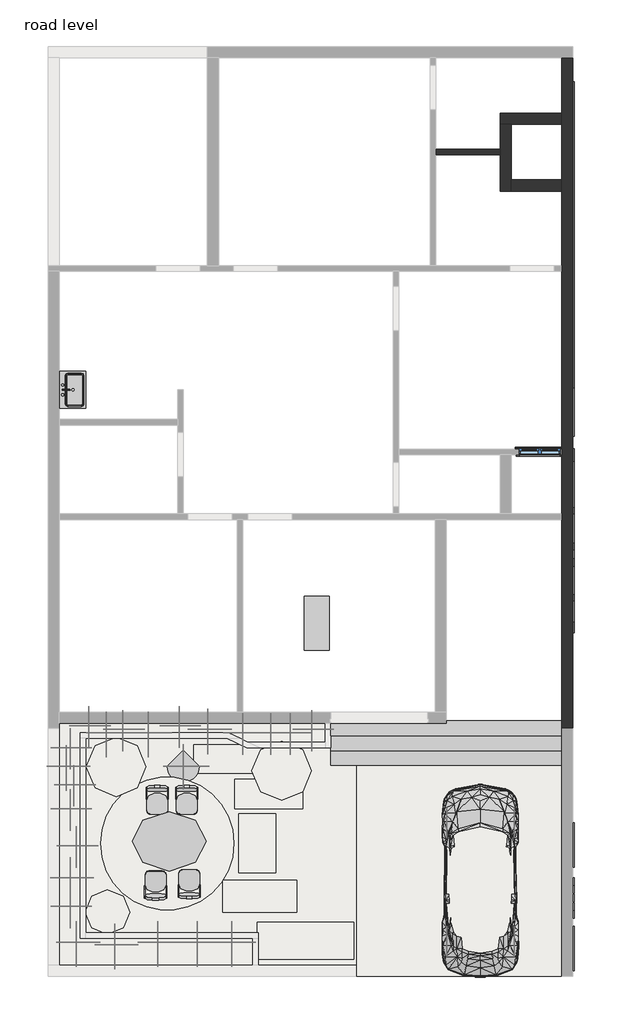
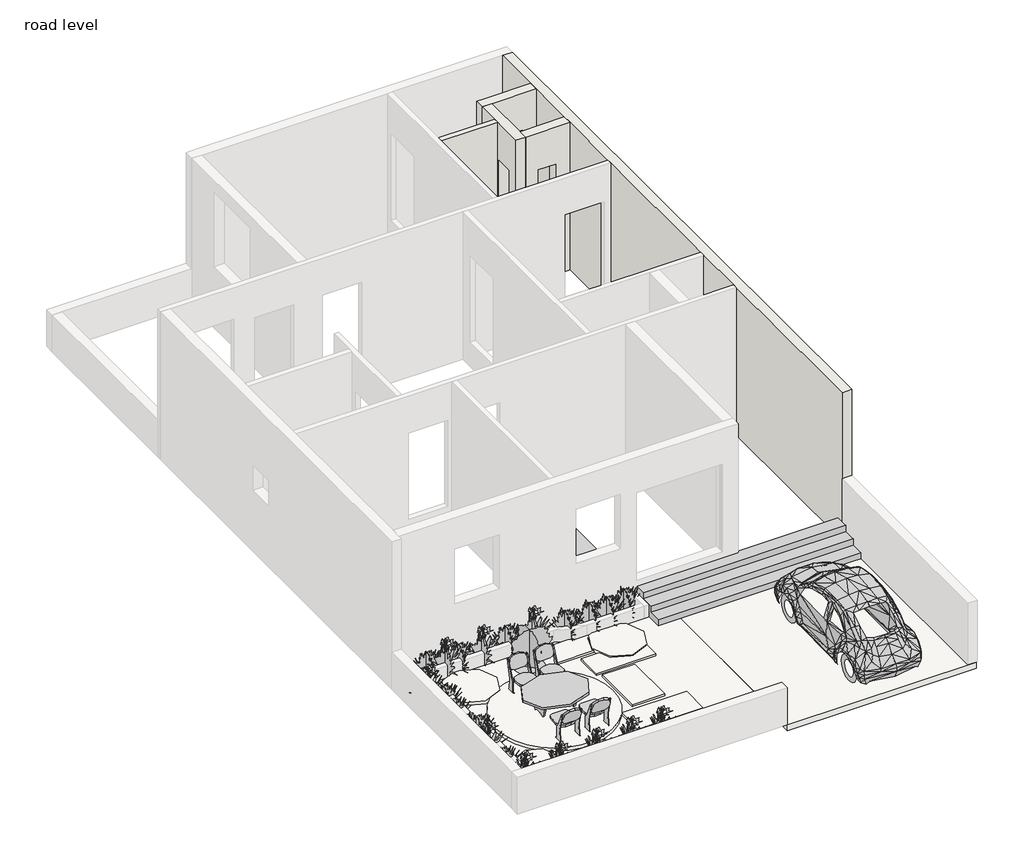
# One storey, part 2 of 2: 23 geographic elements, 9 furniture elements, 7 slabs, 5 proxies, 5 walls, 1 flow terminal, 1 window.
"""IFC4 building model written with IfcOpenShell, lengths in millimetres."""

from ifc_helpers import new_model, si_unit, point, frame, frame_2d, origin, origin_with_axes, place, context, project, spatial, polyline, circle_curve, trimmed, segment, composite_curve, outline, extrude, faceted_brep, transform, mapped, element, save
from components import muntin_pattern_2x2_muntin_pattern_2x2_b3fe6957, muntin_pattern_2x2_muntin_pattern_2x2_3e0ecaf2, rpc_beetle_rpc_beetle_31f8b51e, trim_window_exterior_flat_with_sill_41619996, trim_window_interior_flat_picture_frame_51c85655, flow_terminal_4d548711, casework_1_casework_1_eb7a94e5, casework_2_casework_2_b74305db, casework_3_casework_3_5667240a, furniture_eb3a3c23, furniture_74675f9f, furniture_c105135d, rpc_plant_tropical_55f6ff97, rpc_plant_tropical_dagger_2_80c14bd7, geographic_element_e27c54a3, window_a598f463

model = new_model("IFC4")

# Units and contexts
model_context = context("Model", 3, world=origin())
ifc_project = project(units=[si_unit("LENGTHUNIT", "METRE", prefix="MILLI")], contexts=[model_context])

# Site, building, storey
site = spatial("IfcSite", under=ifc_project)
building = spatial("IfcBuilding", under=site)
storey = spatial("IfcBuildingStorey", under=building, Name="road level", Elevation=0.0)

# Proxies
placement = place(None, origin())
muntin_pattern_2x2_muntin_pattern_2x2_shape = muntin_pattern_2x2_muntin_pattern_2x2_b3fe6957(model_context)
element("IfcBuildingElementProxy", 1, Name="Muntin Pattern_2x2 : Muntin Pattern_2x2", ObjectType="Muntin Pattern_2x2 : Muntin Pattern_2x2", at=placement, inside=storey, context=model_context, shape_type="MappedRepresentation", body=[
    mapped(muntin_pattern_2x2_muntin_pattern_2x2_shape, transform((1784.5376403, 4516.9007925, 984.25), x_axis=(1.0, 0.0, 0.0), y_axis=(0.0, 1.0, 0.0), z_axis=(0.0, 0.0, 1.0))),
])
muntin_pattern_2x2_muntin_pattern_2x2_2_shape = muntin_pattern_2x2_muntin_pattern_2x2_3e0ecaf2(model_context)
element("IfcBuildingElementProxy", 2, Name="Muntin Pattern_2x2 : Muntin Pattern_2x2", ObjectType="Muntin Pattern_2x2 : Muntin Pattern_2x2", at=placement, inside=storey, context=model_context, shape_type="MappedRepresentation", body=[
    mapped(muntin_pattern_2x2_muntin_pattern_2x2_2_shape, transform((2213.1626403, 4516.9007925, 984.25), x_axis=(-1.0, 0.0, 0.0), y_axis=(0.0, -1.0, 0.0), z_axis=(0.0, 0.0, 1.0))),
])
rpc_beetle_rpc_beetle_shape = rpc_beetle_rpc_beetle_31f8b51e(model_context)
element("IfcBuildingElementProxy", 3, Name="RPC Beetle : RPC Beetle", ObjectType="RPC Beetle : RPC Beetle", at=placement, inside=storey, context=model_context, shape_type="MappedRepresentation", body=[
    mapped(rpc_beetle_rpc_beetle_shape, transform((779.6501403, -5586.8025668, 0.0), x_axis=(1.0, 0.0, 0.0), y_axis=(0.0, 1.0, 0.0), z_axis=(0.0, 0.0, 1.0))),
])
trim_window_exterior_flat_with_sill_shape = trim_window_exterior_flat_with_sill_41619996(model_context)
element("IfcBuildingElementProxy", 4, Name="Trim-Window-Exterior-Flat : with Sill", ObjectType="Trim-Window-Exterior-Flat : with Sill", at=placement, inside=storey, context=model_context, shape_type="MappedRepresentation", body=[
    mapped(trim_window_exterior_flat_with_sill_shape, transform((1998.8501403, 4526.4257925, 1828.8), x_axis=(-1.0, 0.0, 0.0), y_axis=(0.0, 0.0, 1.0), z_axis=(0.0, 1.0, 0.0))),
])
trim_window_interior_flat_picture_frame_shape = trim_window_interior_flat_picture_frame_51c85655(model_context)
element("IfcBuildingElementProxy", 5, Name="Trim-Window-Interior-Flat : Picture Frame", ObjectType="Trim-Window-Interior-Flat : Picture Frame", at=placement, inside=storey, context=model_context, shape_type="MappedRepresentation", body=[
    mapped(trim_window_interior_flat_picture_frame_shape, transform((1998.8501403, 4412.1257925, 1828.8), x_axis=(1.0, 0.0, 0.0), y_axis=(0.0, 0.0, 1.0), z_axis=(0.0, -1.0, 0.0))),
])

# Flow terminal
flow_terminal_shape = flow_terminal_4d548711(model_context)
element("IfcFlowTerminal", 6, ObjectType="Sink Kitchen-Single : 30\" x 21\"", at=placement, inside=storey, context=model_context, shape_type="MappedRepresentation", body=[
    mapped(flow_terminal_shape, transform((-7600.0044586, 5729.936552, 0.0), x_axis=(0.0, 1.0, 0.0), y_axis=(-1.0, 0.0, 0.0), z_axis=(0.0, 0.0, 1.0))),
])

# Furniture
casework_1_casework_1_shape = casework_1_casework_1_eb7a94e5(model_context)
element("IfcFurniture", 7, ObjectType="Casework 1 : Casework 1", at=placement, inside=storey, context=model_context, shape_type="MappedRepresentation", body=[
    mapped(casework_1_casework_1_shape, transform((0.0, 0.0, 0.0), x_axis=(1.0, 0.0, 0.0), y_axis=(0.0, 1.0, 0.0), z_axis=(0.0, 0.0, 1.0))),
])
casework_2_casework_2_shape = casework_2_casework_2_b74305db(model_context)
element("IfcFurniture", 8, ObjectType="Casework 2 : Casework 2", at=placement, inside=storey, context=model_context, shape_type="MappedRepresentation", body=[
    mapped(casework_2_casework_2_shape, transform((0.0, 0.0, 0.0), x_axis=(1.0, 0.0, 0.0), y_axis=(0.0, 1.0, 0.0), z_axis=(0.0, 0.0, 1.0))),
])
casework_3_casework_3_shape = casework_3_casework_3_5667240a(model_context)
element("IfcFurniture", 9, ObjectType="Casework 3 : Casework 3", at=placement, inside=storey, context=model_context, shape_type="MappedRepresentation", body=[
    mapped(casework_3_casework_3_shape, transform((0.0, 0.0, 0.0), x_axis=(1.0, 0.0, 0.0), y_axis=(0.0, 1.0, 0.0), z_axis=(0.0, 0.0, 1.0))),
])
furniture_shape = furniture_eb3a3c23(model_context)
element("IfcFurniture", 10, ObjectType="Seating-Auditorium : 18\" x 24\" x 30\"", at=placement, inside=storey, context=model_context, shape_type="MappedRepresentation", body=[
    mapped(furniture_shape, transform((-6061.2777286, -4646.8421746, 76.2), x_axis=(1.0, 0.0, 0.0), y_axis=(0.0, 1.0, 0.0), z_axis=(0.0, 0.0, 1.0))),
])
element("IfcFurniture", 11, ObjectType="Seating-Auditorium : 18\" x 24\" x 30\"", at=placement, inside=storey, context=model_context, shape_type="MappedRepresentation", body=[
    mapped(furniture_shape, transform((-5706.7715198, -2488.6271569, 76.2), x_axis=(-1.0, 0.0, 0.0), y_axis=(0.0, -1.0, 0.0), z_axis=(0.0, 0.0, 1.0))),
])
element("IfcFurniture", 12, ObjectType="Seating-Auditorium : 18\" x 24\" x 30\"", at=placement, inside=storey, context=model_context, shape_type="MappedRepresentation", body=[
    mapped(furniture_shape, transform((-5097.1715198, -2488.6271569, 76.2), x_axis=(-1.0, 0.0, 0.0), y_axis=(0.0, -1.0, 0.0), z_axis=(0.0, 0.0, 1.0))),
])
element("IfcFurniture", 13, ObjectType="Seating-Auditorium : 18\" x 24\" x 30\"", at=placement, inside=storey, context=model_context, shape_type="MappedRepresentation", body=[
    mapped(furniture_shape, transform((-5367.8272575, -4621.4421746, 76.2), x_axis=(1.0, 0.0, 0.0), y_axis=(0.0, 1.0, 0.0), z_axis=(0.0, 0.0, 1.0))),
])
furniture_2_shape = furniture_74675f9f(model_context)
element("IfcFurniture", 14, ObjectType="Table-Coffee Mission : 44\" x 20\"", at=placement, inside=storey, context=model_context, shape_type="MappedRepresentation", body=[
    mapped(furniture_2_shape, transform((-2585.8498597, 945.0257925, 0.0), x_axis=(0.0, 1.0, 0.0), y_axis=(-1.0, 0.0, 0.0), z_axis=(0.0, 0.0, 1.0))),
])
furniture_3_shape = furniture_c105135d(model_context)
element("IfcFurniture", 15, ObjectType="Table-Ellipse : 60\" x 48\"", at=placement, inside=storey, context=model_context, shape_type="MappedRepresentation", body=[
    mapped(furniture_3_shape, transform((-5621.1498597, -3542.5667647, 76.2), x_axis=(1.0, 0.0, 0.0), y_axis=(0.0, 1.0, 0.0), z_axis=(0.0, 0.0, 1.0))),
])

# Geographic elements
rpc_plant_tropical_shape = rpc_plant_tropical_55f6ff97(model_context)
element("IfcGeographicElement", 16, ObjectType="RPC Plant - Tropical", at=placement, inside=storey, context=model_context, shape_type="MappedRepresentation", body=[
    mapped(rpc_plant_tropical_shape, transform((-4330.7993887, -5612.2025668, 0.0), x_axis=(1.0, 0.0, 0.0), y_axis=(0.0, 1.0, 0.0), z_axis=(0.0, 0.0, 1.0))),
])
element("IfcGeographicElement", 17, ObjectType="RPC Plant - Tropical", at=placement, inside=storey, context=model_context, shape_type="MappedRepresentation", body=[
    mapped(rpc_plant_tropical_shape, transform((-5041.9993887, -5612.2025668, 0.0), x_axis=(1.0, 0.0, 0.0), y_axis=(0.0, 1.0, 0.0), z_axis=(0.0, 0.0, 1.0))),
])
element("IfcGeographicElement", 18, ObjectType="RPC Plant - Tropical", at=placement, inside=storey, context=model_context, shape_type="MappedRepresentation", body=[
    mapped(rpc_plant_tropical_shape, transform((-5854.7993887, -5612.2025668, 0.0), x_axis=(1.0, 0.0, 0.0), y_axis=(0.0, 1.0, 0.0), z_axis=(0.0, 0.0, 1.0))),
])
element("IfcGeographicElement", 19, ObjectType="RPC Plant - Tropical", at=placement, inside=storey, context=model_context, shape_type="MappedRepresentation", body=[
    mapped(rpc_plant_tropical_shape, transform((-6743.7993887, -5663.0025668, 0.0), x_axis=(1.0, 0.0, 0.0), y_axis=(0.0, 1.0, 0.0), z_axis=(0.0, 0.0, 1.0))),
])
element("IfcGeographicElement", 20, ObjectType="RPC Plant - Tropical", at=placement, inside=storey, context=model_context, shape_type="MappedRepresentation", body=[
    mapped(rpc_plant_tropical_shape, transform((-7531.1993887, -5612.2025668, 0.0), x_axis=(1.0, 0.0, 0.0), y_axis=(0.0, 1.0, 0.0), z_axis=(0.0, 0.0, 1.0))),
])
element("IfcGeographicElement", 21, ObjectType="RPC Plant - Tropical", at=placement, inside=storey, context=model_context, shape_type="MappedRepresentation", body=[
    mapped(rpc_plant_tropical_shape, transform((-7658.1993887, -4294.0266914, 0.0), x_axis=(1.0, 0.0, 0.0), y_axis=(0.0, 1.0, 0.0), z_axis=(0.0, 0.0, 1.0))),
])
element("IfcGeographicElement", 22, ObjectType="RPC Plant - Tropical", at=placement, inside=storey, context=model_context, shape_type="MappedRepresentation", body=[
    mapped(rpc_plant_tropical_shape, transform((-4827.8987169, -1239.3742075, 0.0), x_axis=(1.0, 0.0, 0.0), y_axis=(0.0, 1.0, 0.0), z_axis=(0.0, 0.0, 1.0))),
])
element("IfcGeographicElement", 23, ObjectType="RPC Plant - Tropical", at=placement, inside=storey, context=model_context, shape_type="MappedRepresentation", body=[
    mapped(rpc_plant_tropical_shape, transform((-6052.9498597, -1309.5266914, 0.0), x_axis=(1.0, 0.0, 0.0), y_axis=(0.0, 1.0, 0.0), z_axis=(0.0, 0.0, 1.0))),
])
element("IfcGeographicElement", 24, ObjectType="RPC Plant - Tropical", at=placement, inside=storey, context=model_context, shape_type="MappedRepresentation", body=[
    mapped(rpc_plant_tropical_shape, transform((-6916.5498597, -1309.5266914, 0.0), x_axis=(1.0, 0.0, 0.0), y_axis=(0.0, 1.0, 0.0), z_axis=(0.0, 0.0, 1.0))),
])
element("IfcGeographicElement", 25, ObjectType="RPC Plant - Tropical", at=placement, inside=storey, context=model_context, shape_type="MappedRepresentation", body=[
    mapped(rpc_plant_tropical_shape, transform((-7734.3993887, -1993.1667647, 0.0), x_axis=(1.0, 0.0, 0.0), y_axis=(0.0, 1.0, 0.0), z_axis=(0.0, 0.0, 1.0))),
])
rpc_plant_tropical_dagger_2_shape = rpc_plant_tropical_dagger_2_80c14bd7(model_context)
element("IfcGeographicElement", 26, ObjectType="RPC Plant - Tropical : Dagger - 2'", at=placement, inside=storey, context=model_context, shape_type="MappedRepresentation", body=[
    mapped(rpc_plant_tropical_dagger_2_shape, transform((-7658.1993887, -4878.2266914, 0.0), x_axis=(1.0, 0.0, 0.0), y_axis=(0.0, 1.0, 0.0), z_axis=(0.0, 0.0, 1.0))),
])
element("IfcGeographicElement", 27, ObjectType="RPC Plant - Tropical : Dagger - 2'", at=placement, inside=storey, context=model_context, shape_type="MappedRepresentation", body=[
    mapped(rpc_plant_tropical_dagger_2_shape, transform((-7531.1993887, -3633.6266914, 0.0), x_axis=(1.0, 0.0, 0.0), y_axis=(0.0, 1.0, 0.0), z_axis=(0.0, 0.0, 1.0))),
])
element("IfcGeographicElement", 28, ObjectType="RPC Plant - Tropical : Dagger - 2'", at=placement, inside=storey, context=model_context, shape_type="MappedRepresentation", body=[
    mapped(rpc_plant_tropical_dagger_2_shape, transform((-7658.1993887, -2871.6266914, 0.0), x_axis=(1.0, 0.0, 0.0), y_axis=(0.0, 1.0, 0.0), z_axis=(0.0, 0.0, 1.0))),
])
element("IfcGeographicElement", 29, ObjectType="RPC Plant - Tropical : Dagger - 2'", at=placement, inside=storey, context=model_context, shape_type="MappedRepresentation", body=[
    mapped(rpc_plant_tropical_dagger_2_shape, transform((-7581.9993887, -2374.1667647, 0.0), x_axis=(1.0, 0.0, 0.0), y_axis=(0.0, 1.0, 0.0), z_axis=(0.0, 0.0, 1.0))),
])
element("IfcGeographicElement", 30, ObjectType="RPC Plant - Tropical : Dagger - 2'", at=placement, inside=storey, context=model_context, shape_type="MappedRepresentation", body=[
    mapped(rpc_plant_tropical_dagger_2_shape, transform((-7658.1993887, -1612.1667647, 0.0), x_axis=(1.0, 0.0, 0.0), y_axis=(0.0, 1.0, 0.0), z_axis=(0.0, 0.0, 1.0))),
])
element("IfcGeographicElement", 31, ObjectType="RPC Plant - Tropical : Dagger - 2'", at=placement, inside=storey, context=model_context, shape_type="MappedRepresentation", body=[
    mapped(rpc_plant_tropical_dagger_2_shape, transform((-7272.1498597, -1163.1742075, 0.0), x_axis=(1.0, 0.0, 0.0), y_axis=(0.0, 1.0, 0.0), z_axis=(0.0, 0.0, 1.0))),
])
element("IfcGeographicElement", 32, ObjectType="RPC Plant - Tropical : Dagger - 2'", at=placement, inside=storey, context=model_context, shape_type="MappedRepresentation", body=[
    mapped(rpc_plant_tropical_dagger_2_shape, transform((-6573.6498597, -1239.3742075, 0.0), x_axis=(1.0, 0.0, 0.0), y_axis=(0.0, 1.0, 0.0), z_axis=(0.0, 0.0, 1.0))),
])
element("IfcGeographicElement", 33, ObjectType="RPC Plant - Tropical : Dagger - 2'", at=placement, inside=storey, context=model_context, shape_type="MappedRepresentation", body=[
    mapped(rpc_plant_tropical_dagger_2_shape, transform((-5417.9498597, -1163.1742075, 0.0), x_axis=(1.0, 0.0, 0.0), y_axis=(0.0, 1.0, 0.0), z_axis=(0.0, 0.0, 1.0))),
])
element("IfcGeographicElement", 34, ObjectType="RPC Plant - Tropical : Dagger - 2'", at=placement, inside=storey, context=model_context, shape_type="MappedRepresentation", body=[
    mapped(rpc_plant_tropical_dagger_2_shape, transform((-4109.8498597, -1309.5266914, 0.0), x_axis=(1.0, 0.0, 0.0), y_axis=(0.0, 1.0, 0.0), z_axis=(0.0, 0.0, 1.0))),
])
element("IfcGeographicElement", 35, ObjectType="RPC Plant - Tropical : Dagger - 2'", at=placement, inside=storey, context=model_context, shape_type="MappedRepresentation", body=[
    mapped(rpc_plant_tropical_dagger_2_shape, transform((-2684.1498597, -1239.3742075, 0.0), x_axis=(1.0, 0.0, 0.0), y_axis=(0.0, 1.0, 0.0), z_axis=(0.0, 0.0, 1.0))),
])
element("IfcGeographicElement", 36, ObjectType="RPC Plant - Tropical : Dagger - 2'", at=placement, inside=storey, context=model_context, shape_type="MappedRepresentation", body=[
    mapped(rpc_plant_tropical_dagger_2_shape, transform((-3126.7726479, -1309.5266914, 0.0), x_axis=(1.0, 0.0, 0.0), y_axis=(0.0, 1.0, 0.0), z_axis=(0.0, 0.0, 1.0))),
])
element("IfcGeographicElement", 37, ObjectType="RPC Plant - Tropical : Dagger - 2'", at=placement, inside=storey, context=model_context, shape_type="MappedRepresentation", body=[
    mapped(rpc_plant_tropical_dagger_2_shape, transform((-3533.1726479, -1309.5266914, 0.0), x_axis=(1.0, 0.0, 0.0), y_axis=(0.0, 1.0, 0.0), z_axis=(0.0, 0.0, 1.0))),
])
geographic_element_shape = geographic_element_e27c54a3(model_context)
element("IfcGeographicElement", 38, ObjectType="RPC Shrub : Cedar Shrub 3'-0\"", at=placement, inside=storey, context=model_context, shape_type="MappedRepresentation", body=[
    mapped(geographic_element_shape, transform((-5329.0498597, -1993.1667647, 76.2), x_axis=(1.0, 0.0, 0.0), y_axis=(0.0, 1.0, 0.0), z_axis=(0.0, 0.0, 1.0))),
])

# Slabs
element("IfcSlab", 39, at=placement, inside=storey, context=model_context, shape_type="SweptSolid", body=[
    extrude(outline(polyline([(-1774.9490674, -1112.3742075), (-1774.9490674, -6090.7742075), (-7881.7498597, -6090.7742075), (-7881.7498597, -1112.3742075), (-1774.9490674, -1112.3742075)])), frame((0.0, 0.0, -152.4), z_axis=(0.0, 0.0, 1.0), x_axis=(1.0, 0.0, 0.0)), (0.0, 0.0, 1.0), 152.4),
])
element("IfcSlab", 40, at=placement, inside=storey, context=model_context, shape_type="SweptSolid", body=[
    extrude(outline(polyline([(2659.2501403, -1112.3742075), (2659.2501403, -6319.3742075), (-1774.9490674, -6319.3742075), (-1774.9490674, -1112.3742075), (2659.2501403, -1112.3742075)])), frame((0.0, 0.0, -152.4), z_axis=(0.0, 0.0, 1.0), x_axis=(1.0, 0.0, 0.0)), (0.0, 0.0, 1.0), 152.4),
])
element("IfcSlab", 41, ObjectType="Generic - 12\"", at=placement, inside=storey, context=model_context, shape_type="SweptSolid", body=[
    extrude(outline(composite_curve([segment(trimmed(circle_curve(frame_2d((-3308.7831315, -2086.2385506)), 609.6), [point((-3918.3831315, -2086.2385506))], [point((-2699.1831315, -2086.2385506))], False, "CARTESIAN"), True, "CONTINUOUS"), segment(trimmed(circle_curve(frame_2d((-3308.7831315, -2086.2385506)), 609.6), [point((-2699.1831315, -2086.2385506))], [point((-3918.3831315, -2086.2385506))], False, "CARTESIAN"), True, "CONTINUOUS")], self_intersect=False)), frame((0.0, 0.0, -228.6), z_axis=(0.0, 0.0, 1.0), x_axis=(1.0, 0.0, 0.0)), (0.0, 0.0, 1.0), 304.8),
])
element("IfcSlab", 42, ObjectType="Generic - 12\"", at=placement, inside=storey, context=model_context, shape_type="SweptSolid", body=[
    extrude(outline(composite_curve([segment(trimmed(circle_curve(frame_2d((-5659.2498597, -3583.8471241)), 1371.6), [point((-7030.8498597, -3583.8471241))], [point((-4287.6498597, -3583.8471241))], False, "CARTESIAN"), True, "CONTINUOUS"), segment(trimmed(circle_curve(frame_2d((-5659.2498597, -3583.8471241)), 1371.6), [point((-4287.6498597, -3583.8471241))], [point((-7030.8498597, -3583.8471241))], False, "CARTESIAN"), True, "CONTINUOUS")], self_intersect=False)), frame((0.0, 0.0, -228.6), z_axis=(0.0, 0.0, 1.0), x_axis=(1.0, 0.0, 0.0)), (0.0, 0.0, 1.0), 304.8),
])
element("IfcSlab", 43, ObjectType="Generic - 12\"", at=placement, inside=storey, context=model_context, shape_type="SweptSolid", body=[
    extrude(outline(composite_curve([segment(trimmed(circle_curve(frame_2d((-6712.3831315, -2010.0385506)), 609.6), [point((-6102.7831315, -2010.0385506))], [point((-7321.9831315, -2010.0385506))], False, "CARTESIAN"), True, "CONTINUOUS"), segment(trimmed(circle_curve(frame_2d((-6712.3831315, -2010.0385506)), 609.6), [point((-7321.9831315, -2010.0385506))], [point((-6102.7831315, -2010.0385506))], False, "CARTESIAN"), True, "CONTINUOUS")], self_intersect=False)), frame((0.0, 0.0, -228.6), z_axis=(0.0, 0.0, 1.0), x_axis=(1.0, 0.0, 0.0)), (0.0, 0.0, 1.0), 304.8),
])
element("IfcSlab", 44, ObjectType="Generic - 12\"", at=placement, inside=storey, context=model_context, shape_type="SweptSolid", body=[
    extrude(outline(composite_curve([segment(trimmed(circle_curve(frame_2d((-6890.1831315, -4994.5734605)), 457.2), [point((-7347.3831315, -4994.5734605))], [point((-6432.9831315, -4994.5734605))], False, "CARTESIAN"), True, "CONTINUOUS"), segment(trimmed(circle_curve(frame_2d((-6890.1831315, -4994.5734605)), 457.2), [point((-6432.9831315, -4994.5734605))], [point((-7347.3831315, -4994.5734605))], False, "CARTESIAN"), True, "CONTINUOUS")], self_intersect=False)), frame((0.0, 0.0, -228.6), z_axis=(0.0, 0.0, 1.0), x_axis=(1.0, 0.0, 0.0)), (0.0, 0.0, 1.0), 304.8),
])
element("IfcSlab", 45, ObjectType="Generic - 12\"", at=placement, inside=storey, context=model_context, shape_type="SweptSolid", body=[
    extrude(outline(polyline([(-3578.3490674, -1548.6667647), (-3578.3490674, -2141.7794103), (-5111.0564513, -2141.7794103), (-5111.0564513, -1548.6667647), (-3578.3490674, -1548.6667647)])), frame((0.0, 0.0, -254.0), z_axis=(0.0, 0.0, 1.0), x_axis=(1.0, 0.0, 0.0)), (0.0, 0.0, 1.0), 304.8),
    extrude(outline(polyline([(-2873.9133698, -2261.4064164), (-2873.9133698, -2871.0064164), (-4270.9133698, -2871.0064164), (-4270.9133698, -2261.4064164), (-2873.9133698, -2261.4064164)])), frame((0.0, 0.0, -254.0), z_axis=(0.0, 0.0, 1.0), x_axis=(1.0, 0.0, 0.0)), (0.0, 0.0, 1.0), 304.8),
    extrude(outline(polyline([(-3425.9490674, -2971.0038882), (-3425.9490674, -4190.2038882), (-4187.9490674, -4190.2038882), (-4187.9490674, -2971.0038882), (-3425.9490674, -2971.0038882)])), frame((0.0, 0.0, -254.0), z_axis=(0.0, 0.0, 1.0), x_axis=(1.0, 0.0, 0.0)), (0.0, 0.0, 1.0), 304.8),
    extrude(outline(polyline([(-2996.3399742, -4340.6167081), (-2996.3399742, -5001.0167081), (-4520.3399742, -5001.0167081), (-4520.3399742, -4340.6167081), (-2996.3399742, -4340.6167081)])), frame((0.0, 0.0, -254.0), z_axis=(0.0, 0.0, 1.0), x_axis=(1.0, 0.0, 0.0)), (0.0, 0.0, 1.0), 304.8),
    extrude(outline(polyline([(-1825.7490674, -5205.8025668), (-1825.7490674, -5967.8025668), (-3806.9490674, -5967.8025668), (-3806.9490674, -5205.8025668), (-1825.7490674, -5205.8025668)])), frame((0.0, 0.0, -254.0), z_axis=(0.0, 0.0, 1.0), x_axis=(1.0, 0.0, 0.0)), (0.0, 0.0, 1.0), 304.8),
])

# Walls
element("IfcWall", 46, at=placement, inside=storey, context=model_context, shape_type="Brep", body=[
    faceted_brep([(2456.0501403, 12578.2257925, 0.0), (2456.0501403, 11435.2257925, 0.0), (2456.0501403, 11206.6257925, 0.0), (2456.0501403, 10063.6257925, 0.0), (2456.0501403, 9835.0257925, 0.0), (2456.0501403, 8298.3257925, 0.0), (2456.0501403, 8184.0257925, 0.0), (2456.0501403, 4526.4257925, 0.0), (2456.0501403, 4412.1257925, 0.0), (2456.0501403, 3192.9257925, 0.0), (2456.0501403, 3078.6257925, 0.0), (2456.0501403, -1213.9742075, 0.0), (2456.0501403, -1213.9742075, 1524.0), (2456.0501403, -1213.9742075, 3657.6), (2456.0501403, -432.9242075, 3657.6), (2456.0501403, 3078.6257925, 3657.6), (2456.0501403, 3192.9257925, 3657.6), (2456.0501403, 4412.1257925, 3657.6), (2456.0501403, 4526.4257925, 3657.6), (2456.0501403, 8184.0257925, 3657.6), (2456.0501403, 8298.3257925, 3657.6), (2456.0501403, 9835.0257925, 3657.6), (2456.0501403, 10063.6257925, 3657.6), (2456.0501403, 11206.6257925, 3657.6), (2456.0501403, 11435.2257925, 3657.6), (2456.0501403, 12578.2257925, 3657.6), (2684.6501403, 12578.2257925, 0.0), (2684.6501403, 12578.2257925, 3657.6), (2684.6501403, -1213.9742075, 3657.6), (2684.6501403, -1213.9742075, 1524.0), (2684.6501403, -1213.9742075, 0.0)], [[[0, 1, 2, 3, 4, 5, 6, 7, 8, 9, 10, 11, 12, 13, 14, 15, 16, 17, 18, 19, 20, 21, 22, 23, 24, 25]], [[26, 27, 28, 29, 30]], [[11, 10, 9, 8, 7, 6, 5, 4, 3, 2, 1, 0, 26, 30]], [[13, 12, 11, 30, 29, 28]], [[0, 25, 27, 26]], [[25, 24, 23, 22, 21, 20, 19, 18, 17, 16, 15, 14, 13, 28, 27]]]),
])
element("IfcWall", 47, at=placement, inside=storey, context=model_context, shape_type="Brep", body=[
    faceted_brep([(2456.0501403, 11435.2257925, 0.0), (1186.0501403, 11435.2257925, 0.0), (1186.0501403, 11435.2257925, 3657.6), (1414.6501403, 11435.2257925, 3657.6), (2456.0501403, 11435.2257925, 3657.6), (1719.4501403, 11435.2257925, 2743.2), (1719.4501403, 11435.2257925, 1524.0), (2125.8501403, 11435.2257925, 1524.0), (2125.8501403, 11435.2257925, 2743.2), (2456.0501403, 11206.6257925, 0.0), (2456.0501403, 11206.6257925, 3657.6), (1414.6501403, 11206.6257925, 3657.6), (1186.0501403, 11206.6257925, 3657.6), (1186.0501403, 11206.6257925, 3200.4), (1186.0501403, 11206.6257925, 0.0), (1414.6501403, 11206.6257925, 0.0), (1719.4501403, 11206.6257925, 2743.2), (2125.8501403, 11206.6257925, 2743.2), (2125.8501403, 11206.6257925, 1524.0), (1719.4501403, 11206.6257925, 1524.0)], [[[0, 1, 2, 3, 4], [5, 6, 7, 8]], [[9, 10, 11, 12, 13, 14, 15], [16, 17, 18, 19]], [[1, 0, 9, 15, 14]], [[0, 4, 10, 9]], [[6, 5, 16, 19]], [[7, 6, 19, 18]], [[8, 7, 18, 17]], [[5, 8, 17, 16]], [[4, 3, 2, 12, 11, 10]], [[1, 14, 13, 12, 2]]]),
])
element("IfcWall", 48, at=placement, inside=storey, context=model_context, shape_type="Brep", body=[
    faceted_brep([(1186.0501403, 11206.6257925, 0.0), (1186.0501403, 10698.6257925, 0.0), (1186.0501403, 10584.3257925, 0.0), (1186.0501403, 9835.0257925, 0.0), (1186.0501403, 9835.0257925, 3657.6), (1186.0501403, 10063.6257925, 3657.6), (1186.0501403, 10584.3257925, 3657.6), (1186.0501403, 10698.6257925, 3657.6), (1186.0501403, 11206.6257925, 3657.6), (1186.0501403, 10127.1257925, 2743.2), (1186.0501403, 10127.1257925, 1524.0), (1186.0501403, 10533.5257925, 1524.0), (1186.0501403, 10533.5257925, 2743.2), (1186.0501403, 10755.7299127, 2743.2), (1186.0501403, 10755.7299127, 1524.0), (1186.0501403, 11162.1299127, 1524.0), (1186.0501403, 11162.1299127, 2743.2), (1414.6501403, 9835.0257925, 0.0), (1414.6501403, 10063.6257925, 0.0), (1414.6501403, 11206.6257925, 0.0), (1414.6501403, 11206.6257925, 3657.6), (1414.6501403, 10063.6257925, 3657.6), (1414.6501403, 9835.0257925, 3657.6), (1414.6501403, 9835.0257925, 3200.4), (1414.6501403, 10127.1257925, 1524.0), (1414.6501403, 10127.1257925, 2743.2), (1414.6501403, 10533.5257925, 2743.2), (1414.6501403, 10533.5257925, 1524.0), (1414.6501403, 10755.7299127, 1524.0), (1414.6501403, 10755.7299127, 2743.2), (1414.6501403, 11162.1299127, 2743.2), (1414.6501403, 11162.1299127, 1524.0)], [[[0, 1, 2, 3, 4, 5, 6, 7, 8], [9, 10, 11, 12], [13, 14, 15, 16]], [[17, 18, 19, 20, 21, 22, 23], [24, 25, 26, 27], [28, 29, 30, 31]], [[3, 2, 1, 0, 19, 18, 17]], [[10, 9, 25, 24]], [[11, 10, 24, 27]], [[12, 11, 27, 26]], [[9, 12, 26, 25]], [[13, 29, 28, 14]], [[14, 28, 31, 15]], [[29, 13, 16, 30]], [[30, 16, 15, 31]], [[20, 8, 7, 6, 5, 4, 22, 21]], [[3, 17, 23, 22, 4]], [[8, 20, 19, 0]]]),
])
element("IfcWall", 49, at=placement, inside=storey, context=model_context, shape_type="SweptSolid", body=[
    extrude(outline(polyline([(3657.6, 1414.6501403), (0.0, 1414.6501403), (0.0, 2456.0501403), (3657.6, 2456.0501403), (3657.6, 1414.6501403)]), holes=[polyline([(2743.2, 2113.1501403), (1524.0, 2113.1501403), (1524.0, 1706.7501403), (2743.2, 1706.7501403), (2743.2, 2113.1501403)])]), frame((0.0, 9835.0257925, 0.0), z_axis=(0.0, 1.0, 0.0), x_axis=(0.0, 0.0, 1.0)), (0.0, 0.0, 1.0), 228.6),
])
element("IfcWall", 50, at=placement, inside=storey, context=model_context, shape_type="SweptSolid", body=[
    extrude(outline(polyline([(-134.7498597, 10698.6257925), (1186.0501403, 10698.6257925), (1186.0501403, 10584.3257925), (-134.7498597, 10584.3257925), (-134.7498597, 10698.6257925)])), origin_with_axes(), (0.0, 0.0, 1.0), 3657.6),
])

# Window
window_shape = window_a598f463(model_context)
element("IfcWindow", 51, ObjectType="Window-Casement-Double : 34\" x 36\"", at=placement, inside=storey, context=model_context, shape_type="MappedRepresentation", body=[
    mapped(window_shape, transform((1998.8501403, 4469.2757925, 0.0), x_axis=(1.0, 0.0, 0.0), y_axis=(0.0, 1.0, 0.0), z_axis=(0.0, 0.0, 1.0))),
])

save(model, "model.ifc")

# Revit data of these elements
# Type "Muntin Pattern_2x2 : Muntin Pattern_2x2"
#   Width [instance default] = 4' - 0"
#   Thickness = 0' - 0 1/2"
#   Height [instance default] = 4' - 0"
#   Distance = 0' - 0 3/4"
#   Interior Material [instance default] = none
#   Exterior Material [instance default] = none
#   Default Elevation = 0
# Type "RPC Beetle : RPC Beetle"
#   built-in parameter 1005198 = "{2, 15},{39, RPC-16-0U6E-L4EG-ENH1-J3KF-SVEL-0TX4-C0},{1, 0},{1, 0},{2, 36},{1, 8},{5, Color},{1, 0},{1, 0},{3, 0.8},{3, 0.8},{3, 0.8},{1, 8},{7, BBoxMin},{1, 0},{1, 0},{1, 0},{1, 0},{1, 0},{1, 8},{7, BBoxMax},{1, 0},{1, 0},{1, 0},{1, 0},{1, 0},{2, 11},{9, RPCTypeId},{1, 0},{1, 0},{39, RPC-16-0U6E-L4EG-ENH1-J3KF-SVEL-0TX4-C0},{1, 6},{14, RPCPlantHeight},{1, 0},{1, 0},{7, 4.91667},{2, 11},{20, AdvancedUIDefinition},{1, 0},{1, 0},{0, },{2, 11},{10, AssetLibID},{1, 0},{1, 0},{36, 4D3F6E72-3F99-4203-98E9-AF80B3C7A7A4},{2, 11},{10, BaseSchema},{1, 0},{1, 0},{9, RPCSchema},{2, 11},{12, ExchangeGUID},{1, 0},{1, 0},{0, },{1, 2},{6, Hidden},{1, 0},{1, 0},{1, 0},{2, 11},{12, LocalizedUID},{1, 0},{1, 0},{0, },{1, 4},{11, RPCCategory},{1, 0},{1, 0},{1, 0},{2, 11},{8, RPCImage},{1, 0},{1, 0},{0, },{1, 4},{13, SchemaVersion},{1, 0},{1, 0},{1, 4},{2, 11},{12, UIDefinition},{1, 0},{1, 0},{0, },{2, 11},{6, UIName},{1, 0},{1, 0},{39, RPC-16-0U6E-L4EG-ENH1-J3KF-SVEL-0TX4-C0},{2, 11},{11, VersionGUID},{1, 0},{1, 0},{9, RPCSchema},{2, 11},{9, assettype},{1, 0},{1, 0},{11, RPCGeometry},{2, 11},{11, description},{1, 0},{1, 0},{0, },{2, 11},{9, localname},{1, 0},{1, 0},{3, RPC},{2, 11},{9, localtype},{1, 0},{1, 0},{3, RPC},{1, 4},{8, revision},{1, 0},{1, 0},{1, 1},{2, 11},{9, thumbnail},{1, 0},{1, 0},{0, },{1, 4},{7, version},{1, 0},{1, 0},{1, 1},{2, 14},{6, Height},{1, 0},{1, 0},{7, 4.91667},{1, 2},{20, RPC_Cast Reflections},{1, 0},{1, 0},{1, 1},{1, 4},{16, RPC_Transparency},{1, 0},{1, 0},{2, 18},{1, 4},{11, RPC_Tinting},{1, 0},{1, 0},{2, 50},{1, 2},{15, RPC_Use Tinting},{1, 0},{1, 0},{1, 0},{1, 2},{17, RPC_License Plate},{1, 0},{1, 0},{1, 0},{2, 11},{25, RPC_License Plate Texture},{1, 0},{1, 0},{64, __RPC:/object data/textures/car/plate/textures/default/rgb/0/0/0},{2, 11},{27, RPC_i_License Plate Texture},{1, 0},{1, 0},{0, },{1, 2},{16, RPC_Custom Plate},{1, 0},{1, 0},{1, 0},{2, 11},{27, RPC_License Plate File Name},{1, 0},{1, 0},{0, },{2, 11},{7, keyword},{1, 0},{1, 0},{27, :Geometry:RPC:VW Beetle [4]},{2, 11},{8, category},{1, 0},{1, 0},{21, :Auto_Economy/Midsize},{21, assetlibrary_base.fbx},{1, 5},"
#   built-in parameter 1005195 = "RPC-16-0U6E-L4EG-ENH1-J3KF-SVEL-0TX4-C0"
#   Height = 0
# Type "Trim-Window-Exterior-Flat : with Sill"
#   Trim Width = 0' - 2 1/4"
#   Trim Thickness_Picture Frame = 0' - 1 1/4"
#   Trim Thickness_with Sill = 0' - 0 3/4"
#   Sill Thickness = 0' - 1 1/4"
#   Opening Width [instance default] = 2' - 0"
#   Opening Height [instance default] = 3' - 0"
#   Default Elevation = 4' - 0"
#   Sill = yes
#   Picture Frame = no
#   Trim Material [instance default] = none
# Type "Trim-Window-Interior-Flat : Picture Frame"
#   Trim Thickness_Picture Frame = 0' - 1 1/4"
#   Trim Width = 0' - 2 1/4"
#   Trim Thickness_with Sill = 0' - 0 3/4"
#   Sill Thickness = 0' - 1 1/4"
#   Opening Width [instance default] = 2' - 0"
#   Opening Height [instance default] = 3' - 0"
#   Default Elevation = 4' - 0"
#   Sill = no
#   Picture Frame = yes
#   Trim Material [instance default] = none
# Type "Sink Kitchen-Single : 30\" x 21\""
#   Assembly Code = "D2010410"
#   Counter Height = 3' - 0"
#   Depth = 1' - 9"
#   Width = 2' - 6"
#   Faucet Material = Steel, Polished
#   Sink Material = Steel, Polished
#   Default Elevation = 0
# Type "Seating-Auditorium : 18\" x 24\" x 30\""
#   Assembly Code = "E2020200"
#   Seat Material = Linen, Beige
#   Frame Material = Steel, Paint Finish, Dark Gray, Matte
#   Default Elevation = 0
# Type "Table-Coffee Mission : 44\" x 20\""
#   Assembly Code = "E2020200"
#   Height = 1' - 5"
#   Length = 3' - 8"
#   Width = 1' - 8"
#   Material = Wood - Mahogany
#   Default Elevation = 0
# Type "Table-Ellipse : 60\" x 48\""
#   Assembly Code = "E2020200"
#   Half Width = 2' - 0"
#   Half Length = 2' - 6"
#   Height = 1' - 6"
#   Length = 5' - 0"
#   Width = 4' - 0"
#   Base Material = Birch
#   Top Material = Birch
#   Default Elevation = 0
# Type "RPC Plant - Tropical"
#   built-in parameter 1005198 = "{2, 15},{39, RPC-16-FWM5-GM7X-C67P-4000-ST1L-LVER-AU},{1, 0},{1, 0},{2, 35},{1, 8},{5, Color},{1, 0},{1, 0},{3, 0.8},{3, 0.8},{3, 0.8},{1, 8},{7, BBoxMin},{1, 0},{1, 0},{1, 0},{1, 0},{1, 0},{1, 8},{7, BBoxMax},{1, 0},{1, 0},{1, 0},{1, 0},{1, 0},{2, 11},{9, RPCTypeId},{1, 0},{1, 0},{39, RPC-16-FWM5-GM7X-C67P-4000-ST1L-LVER-AU},{1, 6},{14, RPCPlantHeight},{1, 0},{1, 0},{1, 3},{2, 11},{7, keyword},{1, 0},{1, 0},{99, :Geometry:RPC:Crane Lily:strelitzia:reinae:crane lily:plants:shrub:flower:tropical:bird-of-paradise},{2, 11},{8, category},{1, 0},{1, 0},{17, :Shrubs [General]},{2, 11},{12, LocalizedUID},{1, 0},{1, 0},{10, Crane Lily},{2, 14},{6, Height},{1, 0},{1, 0},{1, 3},{1, 2},{16, Cast Reflections},{1, 0},{1, 0},{1, 0},{1, 2},{12, Cast Shadows},{1, 0},{1, 0},{1, 1},{1, 2},{9, Lock View},{1, 0},{1, 0},{1, 0},{1, 4},{5, ViewC},{1, 0},{1, 0},{1, 0},{2, 11},{20, AdvancedUIDefinition},{1, 0},{1, 0},{0, },{2, 11},{10, AssetLibID},{1, 0},{1, 0},{36, 4D3F6E72-3F99-4203-98E9-AF80B3C7A7A4},{2, 11},{10, BaseSchema},{1, 0},{1, 0},{9, RPCSchema},{2, 11},{12, ExchangeGUID},{1, 0},{1, 0},{0, },{1, 2},{6, Hidden},{1, 0},{1, 0},{1, 0},{1, 4},{11, RPCCategory},{1, 0},{1, 0},{1, 0},{2, 11},{8, RPCImage},{1, 0},{1, 0},{0, },{1, 4},{13, SchemaVersion},{1, 0},{1, 0},{1, 4},{2, 11},{12, UIDefinition},{1, 0},{1, 0},{0, },{2, 11},{6, UIName},{1, 0},{1, 0},{39, RPC-16-FWM5-GM7X-C67P-4000-ST1L-LVER-AU},{2, 11},{11, VersionGUID},{1, 0},{1, 0},{9, RPCSchema},{2, 11},{9, assettype},{1, 0},{1, 0},{11, RPCGeometry},{2, 11},{11, description},{1, 0},{1, 0},{0, },{2, 11},{9, localname},{1, 0},{1, 0},{3, RPC},{2, 11},{9, localtype},{1, 0},{1, 0},{3, RPC},{1, 4},{8, revision},{1, 0},{1, 0},{1, 1},{2, 11},{9, thumbnail},{1, 0},{1, 0},{0, },{1, 4},{7, version},{1, 0},{1, 0},{1, 1},{1, 2},{20, RPC_Cast Reflections},{1, 0},{1, 0},{1, 1},{1, 2},{16, RPC_Cast Shadows},{1, 0},{1, 0},{1, 1},{1, 2},{13, RPC_Lock View},{1, 0},{1, 0},{1, 0},{1, 4},{9, RPC_ViewC},{1, 0},{1, 0},{1, 0},{21, assetlibrary_base.fbx},{1, 5},"
#   built-in parameter 1005195 = "RPC-16-FWM5-GM7X-C67P-4000-ST1L-LVER-AU"
#   Assembly Code = "G2050500"
#   Height = 3' - 0"
#   Default Elevation = 0
# Type "RPC Plant - Tropical : Dagger - 2'"
#   built-in parameter 1005198 = "{2, 15},{39, RPC-16-G3A7-NEG0-UH6H-J000-ST1L-LVER-AU},{1, 0},{1, 0},{2, 35},{1, 8},{5, Color},{1, 0},{1, 0},{3, 0.8},{3, 0.8},{3, 0.8},{1, 8},{7, BBoxMin},{1, 0},{1, 0},{1, 0},{1, 0},{1, 0},{1, 8},{7, BBoxMax},{1, 0},{1, 0},{1, 0},{1, 0},{1, 0},{2, 11},{9, RPCTypeId},{1, 0},{1, 0},{39, RPC-16-G3A7-NEG0-UH6H-J000-ST1L-LVER-AU},{1, 6},{14, RPCPlantHeight},{1, 0},{1, 0},{1, 2},{2, 11},{7, keyword},{1, 0},{1, 0},{55, :Geometry:RPC:Dagger:Yucca Recurvifolia:plant:tropical.},{2, 11},{8, category},{1, 0},{1, 0},{17, :Plants [General]},{2, 11},{12, LocalizedUID},{1, 0},{1, 0},{6, Dagger},{2, 14},{6, Height},{1, 0},{1, 0},{1, 2},{1, 2},{16, Cast Reflections},{1, 0},{1, 0},{1, 0},{1, 2},{12, Cast Shadows},{1, 0},{1, 0},{1, 1},{1, 2},{9, Lock View},{1, 0},{1, 0},{1, 0},{1, 4},{5, ViewC},{1, 0},{1, 0},{1, 0},{2, 11},{20, AdvancedUIDefinition},{1, 0},{1, 0},{0, },{2, 11},{10, AssetLibID},{1, 0},{1, 0},{36, 4D3F6E72-3F99-4203-98E9-AF80B3C7A7A4},{2, 11},{10, BaseSchema},{1, 0},{1, 0},{9, RPCSchema},{2, 11},{12, ExchangeGUID},{1, 0},{1, 0},{0, },{1, 2},{6, Hidden},{1, 0},{1, 0},{1, 0},{1, 4},{11, RPCCategory},{1, 0},{1, 0},{1, 0},{2, 11},{8, RPCImage},{1, 0},{1, 0},{0, },{1, 4},{13, SchemaVersion},{1, 0},{1, 0},{1, 4},{2, 11},{12, UIDefinition},{1, 0},{1, 0},{0, },{2, 11},{6, UIName},{1, 0},{1, 0},{39, RPC-16-G3A7-NEG0-UH6H-J000-ST1L-LVER-AU},{2, 11},{11, VersionGUID},{1, 0},{1, 0},{9, RPCSchema},{2, 11},{9, assettype},{1, 0},{1, 0},{11, RPCGeometry},{2, 11},{11, description},{1, 0},{1, 0},{0, },{2, 11},{9, localname},{1, 0},{1, 0},{3, RPC},{2, 11},{9, localtype},{1, 0},{1, 0},{3, RPC},{1, 4},{8, revision},{1, 0},{1, 0},{1, 1},{2, 11},{9, thumbnail},{1, 0},{1, 0},{0, },{1, 4},{7, version},{1, 0},{1, 0},{1, 1},{1, 2},{20, RPC_Cast Reflections},{1, 0},{1, 0},{1, 1},{1, 2},{16, RPC_Cast Shadows},{1, 0},{1, 0},{1, 1},{1, 2},{13, RPC_Lock View},{1, 0},{1, 0},{1, 0},{1, 4},{9, RPC_ViewC},{1, 0},{1, 0},{1, 0},{21, assetlibrary_base.fbx},{1, 5},"
#   built-in parameter 1005195 = "RPC-16-G3A7-NEG0-UH6H-J000-ST1L-LVER-AU"
#   Type Comments = "Dagger"
#   Assembly Code = "G2050500"
#   Height = 2' - 0"
#   Default Elevation = 0
# Type "RPC Shrub : Cedar Shrub 3'-0\""
#   Type Comments = "Cedar Shrub"
#   built-in parameter 1005198 = "{2, 15},{39, RPC-16-FUMD-ULXX-U7X6-J000-ST1L-LVER-AU},{1, 0},{1, 0},{2, 35},{1, 8},{5, Color},{1, 0},{1, 0},{3, 0.8},{3, 0.8},{3, 0.8},{1, 8},{7, BBoxMin},{1, 0},{1, 0},{1, 0},{1, 0},{1, 0},{1, 8},{7, BBoxMax},{1, 0},{1, 0},{1, 0},{1, 0},{1, 0},{2, 11},{9, RPCTypeId},{1, 0},{1, 0},{39, RPC-16-FUMD-ULXX-U7X6-J000-ST1L-LVER-AU},{1, 6},{14, RPCPlantHeight},{1, 0},{1, 0},{1, 3},{2, 11},{7, keyword},{1, 0},{1, 0},{158, :Geometry:RPC:Cedar Shrub:Little Bush:cedar:miniature:evergreen:conifer:shrub:eastern red cedar:juniper:hedge:juniperus virginiana:genevrier de virginie:thuja},{2, 11},{8, category},{1, 0},{1, 0},{17, :Shrubs [General]},{2, 11},{12, LocalizedUID},{1, 0},{1, 0},{11, Cedar Shrub},{2, 14},{6, Height},{1, 0},{1, 0},{1, 3},{1, 2},{16, Cast Reflections},{1, 0},{1, 0},{1, 0},{1, 2},{12, Cast Shadows},{1, 0},{1, 0},{1, 1},{1, 2},{9, Lock View},{1, 0},{1, 0},{1, 0},{1, 4},{5, ViewC},{1, 0},{1, 0},{1, 0},{2, 11},{20, AdvancedUIDefinition},{1, 0},{1, 0},{0, },{2, 11},{10, AssetLibID},{1, 0},{1, 0},{36, 4D3F6E72-3F99-4203-98E9-AF80B3C7A7A4},{2, 11},{10, BaseSchema},{1, 0},{1, 0},{9, RPCSchema},{2, 11},{12, ExchangeGUID},{1, 0},{1, 0},{0, },{1, 2},{6, Hidden},{1, 0},{1, 0},{1, 0},{1, 4},{11, RPCCategory},{1, 0},{1, 0},{1, 0},{2, 11},{8, RPCImage},{1, 0},{1, 0},{0, },{1, 4},{13, SchemaVersion},{1, 0},{1, 0},{1, 4},{2, 11},{12, UIDefinition},{1, 0},{1, 0},{0, },{2, 11},{6, UIName},{1, 0},{1, 0},{39, RPC-16-FUMD-ULXX-U7X6-J000-ST1L-LVER-AU},{2, 11},{11, VersionGUID},{1, 0},{1, 0},{9, RPCSchema},{2, 11},{9, assettype},{1, 0},{1, 0},{11, RPCGeometry},{2, 11},{11, description},{1, 0},{1, 0},{0, },{2, 11},{9, localname},{1, 0},{1, 0},{3, RPC},{2, 11},{9, localtype},{1, 0},{1, 0},{3, RPC},{1, 4},{8, revision},{1, 0},{1, 0},{1, 1},{2, 11},{9, thumbnail},{1, 0},{1, 0},{0, },{1, 4},{7, version},{1, 0},{1, 0},{1, 1},{1, 2},{20, RPC_Cast Reflections},{1, 0},{1, 0},{1, 1},{1, 2},{16, RPC_Cast Shadows},{1, 0},{1, 0},{1, 1},{1, 2},{13, RPC_Lock View},{1, 0},{1, 0},{1, 0},{1, 4},{9, RPC_ViewC},{1, 0},{1, 0},{1, 0},{21, assetlibrary_base.fbx},{1, 5},"
#   built-in parameter 1005195 = "RPC-16-FUMD-ULXX-U7X6-J000-ST1L-LVER-AU"
#   Assembly Code = "G2050500"
#   Height = 3' - 0"
#   Default Elevation = 0
# Type
#   Assembly Code = "B1010"
#   Function = 0
#   Layers, outside or top first: 0' - 6" "Concrete, Cast-in-Place gray" (function 1)
# Type "Generic - 12\""
#   Assembly Code = "B1010"
#   Function = 0
#   Layers, outside or top first: 1' - 0" "Concrete, Cast-in-Place gray" (function 1)
# Type
#   Assembly Code = "B2010"
#   Layers, outside or top first: 0' - 9" no material (function 1)
# Type
#   Assembly Code = "B2010"
#   Layers, outside or top first: 0' - 4 1/2" no material (function 1)
# Type "Window-Casement-Double : 34\" x 36\""
#   Type Mark = "14"
#   Fire Rating = "0.5h"
#   Assembly Code = "B2020100"
#   Analytic Construction = "Double glazing - domestic"
#   Frame Extension [instance default] = 0' - 0 1/4"
#   Window Inset [instance default] = 0' - 0"
#   Wall Thickness [instance default] = 0' - 6"
#   Interior Wall Closure [instance default] = 0' - 2 1/4"
#   Half Width = 1' - 5"
#   Visual Light Transmittance = 0.81
#   Thermal Resistance (R) = 1.8146 (h·ft²·°F)/BTU
#   Solar Heat Gain Coefficient = 0.76
#   Rough Width = 2' - 10 1/2"
#   Rough Height = 3' - 0 1/2"
#   Height = 3' - 0"
#   Heat Transfer Coefficient (U) = 0.5511 BTU/(h·ft²·°F)
#   Exterior Wall Closure [instance default] = 0' - 1 1/4"
#   Extension Jamb [instance default] = 0' - 2 1/4"
#   Default Sill Height = 3' - 0"
#   Width = 2' - 10"
#   Define Thermal Properties by = 0
#   Muntin Visibility = yes
#   Interior Trim Visibility [instance default] = yes
#   Exterior Trim Visibility [instance default] = yes
#   Extension Jamb Visibility [instance default] = yes
#   Interior Trim Material = Wood - Stained
#   Muntin Pattern = Muntin Pattern_2x2 : Muntin Pattern_2x2
#   Interior Trim = Trim-Window-Interior-Flat : Picture Frame
#   Interior Frame Material = Wood - Stained
#   Glass Panel Material = Glass
#   Exterior Trim Material = Clad - White
#   Exterior Trim = Trim-Window-Exterior-Flat : with Sill
#   Exterior Frame Material = Clad - White
#   Wall Closure = (empty or 0)
# Elements 1, 2 (IfcBuildingElementProxy, "Muntin Pattern_2x2 : Muntin Pattern_2x2")
#   Width = 0' - 11 5/8"
#   Height = 2' - 6 1/2"
#   Interior Material = Wood - Stained
#   Exterior Material = Clad - White
#   Phase Created = New Construction
#   Materials on its faces: "Clad - White", "Wood - Stained"
# Element 3 (IfcBuildingElementProxy, "RPC Beetle : RPC Beetle")
#   Phase Created = New Construction
# Element 4 (IfcBuildingElementProxy, "Trim-Window-Exterior-Flat : with Sill")
#   Opening Width = 2' - 10"
#   Opening Height = 3' - 0"
#   Trim Material = Clad - White
#   Phase Created = New Construction
#   Materials on its faces: "Clad - White"
# Element 5 (IfcBuildingElementProxy, "Trim-Window-Interior-Flat : Picture Frame")
#   Opening Width = 2' - 10"
#   Opening Height = 3' - 0"
#   Trim Material = Wood - Stained
#   Phase Created = New Construction
#   Materials on its faces: "Wood - Stained"
# Element 6 (IfcFlowTerminal, "Sink Kitchen-Single : 30\" x 21\"")
#   Mark = "6"
#   Phase Created = New Construction
#   Materials on its faces: "Steel, Polished"
# Element 7 (IfcFurniture, "Casework 1 : Casework 1")
#   Phase Created = New Construction
#   Materials on its faces: "Asphalt Shingle"
# Element 8 (IfcFurniture, "Casework 2 : Casework 2")
#   Phase Created = New Construction
#   Materials on its faces: "Clad - White"
# Element 9 (IfcFurniture, "Casework 3 : Casework 3")
#   Phase Created = New Construction
#   Materials on its faces: "Laminate, Ivory, Matte"
# Elements 10, 11, 12, 13 (IfcFurniture, "Seating-Auditorium : 18\" x 24\" x 30\"")
#   Phase Created = New Construction
#   Materials on its faces: "Steel, Paint Finish, Dark Gray, Matte", "Linen, Beige"
# Element 14 (IfcFurniture, "Table-Coffee Mission : 44\" x 20\"")
#   Phase Created = New Construction
#   Materials on its faces: "Wood - Mahogany"
# Element 15 (IfcFurniture, "Table-Ellipse : 60\" x 48\"")
#   Phase Created = New Construction
#   Materials on its faces: "Birch"
# Elements 16, 17, 18, 19, 20, 21, 22, 23, 24, 25 (IfcGeographicElement, "RPC Plant - Tropical")
#   Phase Created = New Construction
# Elements 26, 27, 28, 29, 30, 31, 32, 33, 34, 35, 36, 37 (IfcGeographicElement, "RPC Plant - Tropical : Dagger - 2'")
#   Phase Created = New Construction
# Element 38 (IfcGeographicElement, "RPC Shrub : Cedar Shrub 3'-0\"")
#   Phase Created = New Construction
# Element 39 (IfcSlab)
#   Height Offset From Level = 0' - 0"
#   Phase Created = New Construction
#   Materials on its faces: "Concrete, Cast-in-Place gray", "Earth"
# Element 40 (IfcSlab)
#   Height Offset From Level = 0' - 0"
#   Phase Created = New Construction
#   Materials on its faces: "Concrete, Cast-in-Place gray"
# Elements 41, 42, 43, 44 (IfcSlab, "Generic - 12\"")
#   Height Offset From Level = 0' - 3"
#   Phase Created = New Construction
#   Materials on its faces: "Grass", "Concrete, Cast-in-Place gray"
# Element 45 (IfcSlab, "Generic - 12\"")
#   Height Offset From Level = 0' - 2"
#   Phase Created = New Construction
#   Materials on its faces: "Concrete, Cast-in-Place gray"
# Element 46 (IfcWall)
#   Top Offset = 0' - 0"
#   Base Offset = 0' - 0"
#   wall height = 12' - 0"
#   Phase Created = New Construction
#   Base Constraint = road level
#   Top Constraint = 2nd floor
#   Materials on its faces: "Default Wall"
# Elements 47, 48, 49, 50 (IfcWall)
#   Top Offset = 0' - 0"
#   Base Offset = 0' - 0"
#   wall height = 12' - 0"
#   Phase Created = New Construction
#   Base Constraint = road level
#   Top Constraint = 1st floor
#   Materials on its faces: "Default Wall"
# Element 51 (IfcWindow, "Window-Casement-Double : 34\" x 36\"")
#   Mark = "10"
#   Window Inset = 0' - 0"
#   Interior Wall Closure = 0' - 2 1/4"
#   Frame Extension = 0' - 0 1/4"
#   Exterior Wall Closure = 0' - 1 1/4"
#   Interior Trim Visibility = yes
#   Exterior Trim Visibility = yes
#   Phase Created = New Construction
#   Materials on its faces: "Wood - Stained", "Glass", "Clad - White"
# Materials
#   "Steel, Polished": class "Metal", colour RGB 57 57 57, transparency 0, Description = "Polished steel", Cost = 0
#   "Linen, Beige": class "Textile", colour RGB 249 239 230, transparency 0, Description = "Linen, beige", Cost = 0
#   "Steel, Paint Finish, Dark Gray, Matte": class "Metal", colour RGB 0 0 0, transparency 0, Description = "Steel, paint finish, dark gray, matte", Cost = 0
#   "Wood - Mahogany": colour RGB 138 86 45, transparency 0
#   "Birch": class "Wood", colour RGB 224 178 126, transparency 0, Description = "Betula Alleghaniensis", Cost = 0
#   "Concrete, Cast-in-Place gray": class "Concrete", colour RGB 192 192 192, transparency 0, Description = "Cast-in-place concrete", Cost = 0
#   "Wood - Stained": class "Wood", colour RGB 224 178 126, transparency 0, Cost = 0
#   "Glass": class "Glass", colour RGB 0 128 192, transparency 0.75, Description = "Soda Lime Glass", Cost = 0
#   "Clad - White": class "Wood", colour RGB 242 242 238, transparency 0, Cost = 0
#   "Asphalt Shingle": class "Generic", colour RGB 155 155 155, transparency 0, Description = "Asphalt roofing shingle", Cost = 0
#   "Laminate, Ivory, Matte": class "Plastic", colour RGB 247 247 239, transparency 0, Description = "Plastic Laminate - Ivory, Matte", Cost = 0
#   "Earth": class "Generic", colour RGB 97 75 62, transparency 0, Description = "Soil", Cost = 0
#   "Grass": class "Generic", colour RGB 104 137 66, transparency 0, Description = "Physical material.", Cost = 0
#   "Default Wall": colour RGB 128 128 128, transparency 0, Cost = 0
